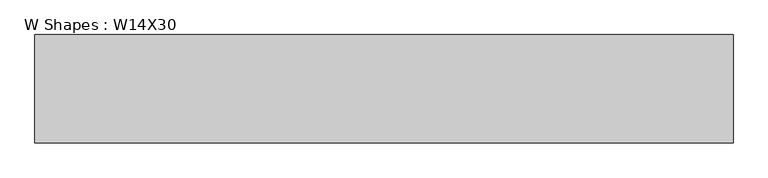
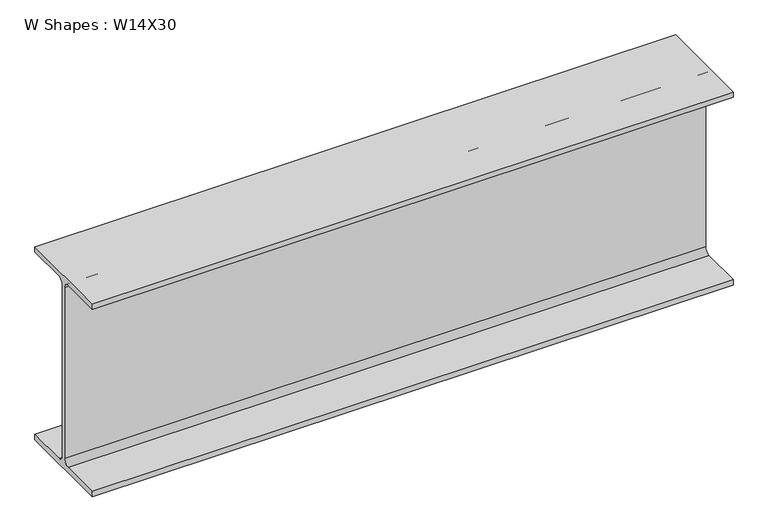
"""IFC4 building model written with IfcOpenShell, lengths in millimetres: beam geometry, W Shapes : W14X30."""

from ifc_helpers import new_model, si_unit, point, frame, frame_2d, origin, place, context, project, spatial, polyline, circle_curve, trimmed, segment, composite_curve, outline, extrude, source, transform, mapped, element, save


def w_shapes_w14x30_b44ec7f2(model_context):
    return source(origin(), model_context, "Body", "SweptSolid", [
        extrude(outline(composite_curve([segment(polyline([(85.471, -165.481), (85.471, -175.26), (-85.471, -175.26), (-85.471, -165.481), (-13.589, -165.481)]), True, "CONTINUOUS"), segment(trimmed(circle_curve(frame_2d((-13.589, -155.321)), 10.16), [point((-13.589, -165.481))], [point((-3.429, -155.321))], True, "CARTESIAN"), True, "CONTINUOUS"), segment(polyline([(-3.429, -155.321), (-3.429, 155.321)]), True, "CONTINUOUS"), segment(trimmed(circle_curve(frame_2d((-13.589, 155.321)), 10.16), [point((-3.429, 155.321))], [point((-13.589, 165.481))], True, "CARTESIAN"), True, "CONTINUOUS"), segment(polyline([(-13.589, 165.481), (-85.471, 165.481), (-85.471, 175.26), (85.471, 175.26), (85.471, 165.481), (13.589, 165.481)]), True, "CONTINUOUS"), segment(trimmed(circle_curve(frame_2d((13.589, 155.321)), 10.16), [point((13.589, 165.481))], [point((3.429, 155.321))], True, "CARTESIAN"), True, "CONTINUOUS"), segment(polyline([(3.429, 155.321), (3.429, -155.321)]), True, "CONTINUOUS"), segment(trimmed(circle_curve(frame_2d((13.589, -155.321)), 10.16), [point((3.429, -155.321))], [point((13.589, -165.481))], True, "CARTESIAN"), True, "CONTINUOUS"), segment(polyline([(13.589, -165.481), (85.471, -165.481)]), True, "CONTINUOUS")], self_intersect=False)), frame((-574.04, 0.0, 0.0), z_axis=(1.0, 0.0, 0.0), x_axis=(0.0, 1.0, 0.0)), (0.0, 0.0, 1.0), 1100.2095299),
    ])


if __name__ == "__main__":
    model = new_model("IFC4")
    model_context = context("Model", 3, world=origin())
    ifc_project = project(units=[si_unit("LENGTHUNIT", "METRE", prefix="MILLI")], contexts=[model_context])
    site = spatial("IfcSite", under=ifc_project)
    building = spatial("IfcBuilding", under=site)
    placement = place(None, origin())
    w_shapes_w14x30_shape = w_shapes_w14x30_b44ec7f2(model_context)
    element("IfcBeam", 1, ObjectType="W Shapes : W14X30", at=placement, inside=building, context=model_context, shape_type="MappedRepresentation", body=[
        mapped(w_shapes_w14x30_shape, transform((0.0, 0.0, 0.0), x_axis=(1.0, 0.0, 0.0), y_axis=(0.0, 1.0, 0.0), z_axis=(0.0, 0.0, 1.0))),
    ])
    save(model, "model.ifc")

# Revit data of these elements
# Type "W Shapes : W14X30"
#   Section Name Key = "W14X30"
#   Width = 6.730"
#   Web Thickness = 0.270"
#   Web Fillet = 0.400"
#   Warping Constant = 887.00 in⁶
#   Torsional Moment of Inertia = 0.38 in⁴
#   Section Area = 8.85 in²
#   Plastic Modulus weak axis = 8.99 in³
#   Plastic Modulus strong axis = 47.30 in³
#   Perimeter = 4.441 ft²/ft
#   Nominal Weight = 30.00 lbf/ft
#   Moment of Inertia weak axis = 19.60 in⁴
#   Moment of Inertia strong axis = 291.00 in⁴
#   Height = 13.800"
#   Flange Thickness = 0.385"
#   Elastic Modulus weak axis = 5.82 in³
#   Elastic Modulus strong axis = 42.00 in³
#   Clear Web Height = 0' - 11 5/8"
#   Centroid Vertical = 6.900"
#   Centroid Horizontal = 3.365"
#   Bolt Spacing = 0' - 3 1/2"
#   Length [instance default] = 1524 mm
#   Structural Material [instance default] = Steel ASTM A992
#   Principal Axes Angle = 0
# Element 1 (IfcBeam, "W Shapes : W14X30")
#   Materials on its faces: "Steel ASTM A992"
# Materials
#   "Steel ASTM A992": class "Metal", colour RGB 199 199 199, transparency 0, Description = "Structural steel 50ksi", Cost = 0
